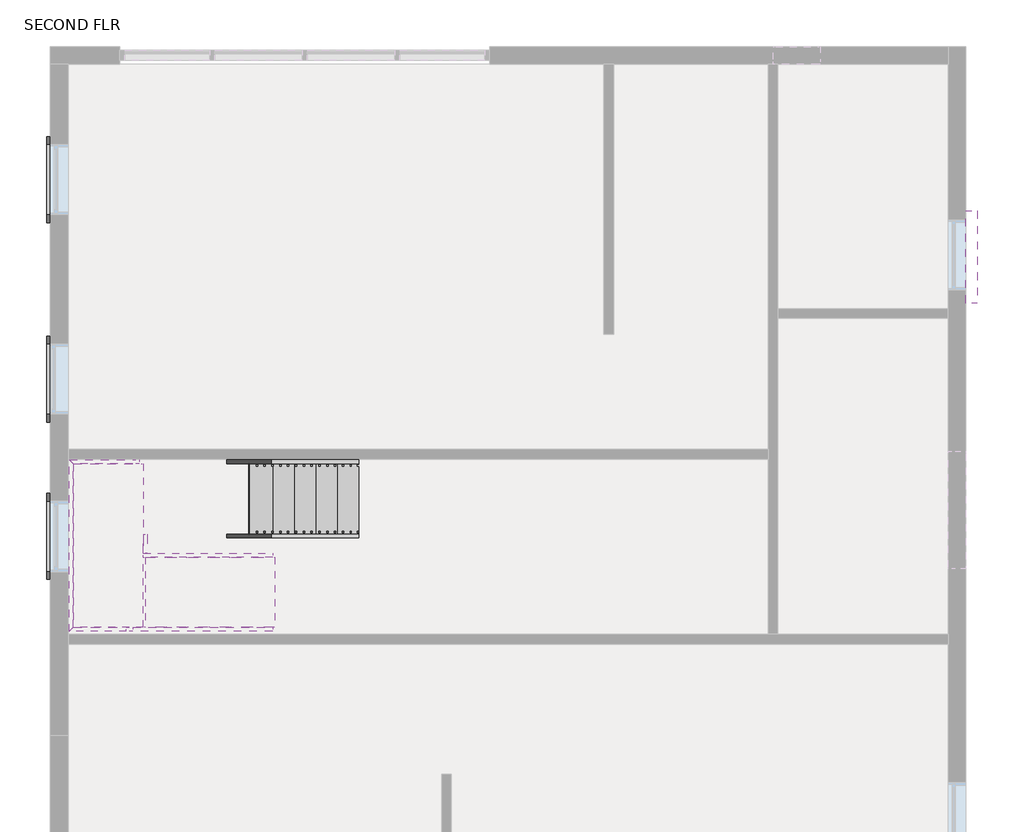
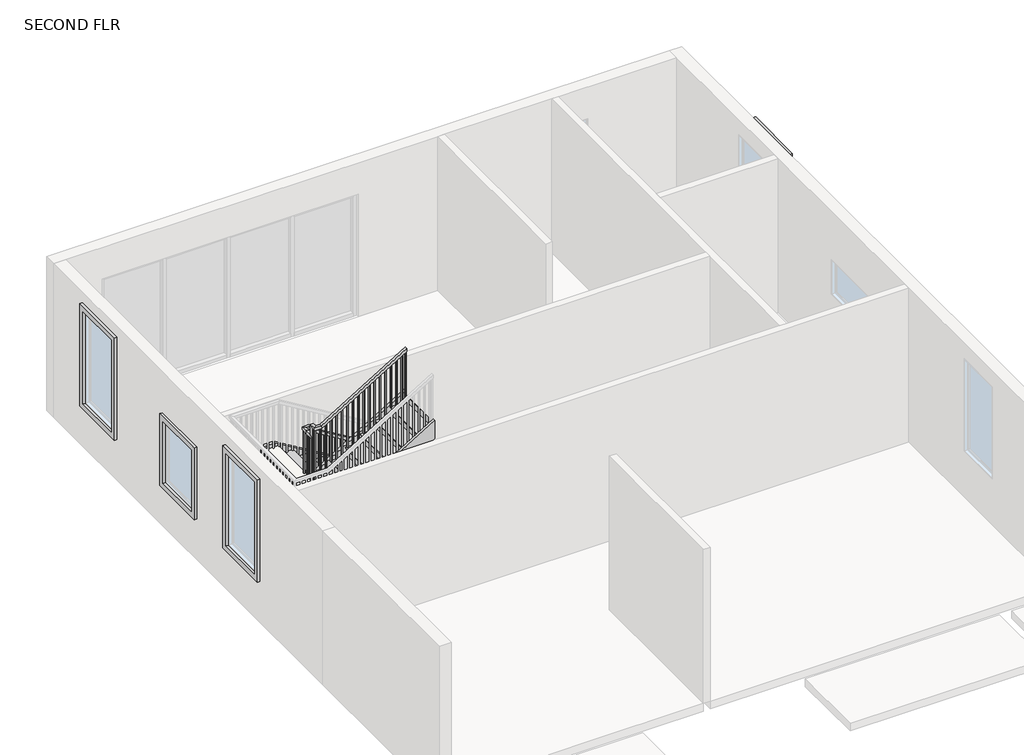
# One storey, part 3 of 3: 8 members, 4 proxies, 2 stair flights, 1 railing, 1 slab.
"""IFC4 building model written with IfcOpenShell, lengths in millimetres."""

from ifc_helpers import new_model, si_unit, frame, origin, place, context, project, spatial, polyline, outline, extrude, faceted_brep, transform, mapped, element, save
from components import generic_models_14_generic_models_13_4ffb657b, generic_models_21_generic_models_23_029173b4, generic_models_24_generic_models_24_8205a677, non_monolithic_landing_255cec53, stair_flight_4502834e, stair_flight_848efa21

model = new_model("IFC4")

# Units and contexts
model_context = context("Model", 3, world=origin())
ifc_project = project(units=[si_unit("LENGTHUNIT", "METRE", prefix="MILLI")], contexts=[model_context])

# Site, building, storey
site = spatial("IfcSite", under=ifc_project)
building = spatial("IfcBuilding", under=site)
storey = spatial("IfcBuildingStorey", under=building, Name="SECOND FLR", Elevation=6400.8)

# Proxies
placement = place(None, origin())
generic_models_14_generic_models_13_shape = generic_models_14_generic_models_13_4ffb657b(model_context)
element("IfcBuildingElementProxy", 1, Name="Generic Models 14 : Generic Models 13", ObjectType="Generic Models 14 : Generic Models 13", at=placement, inside=storey, context=model_context, shape_type="MappedRepresentation", body=[
    mapped(generic_models_14_generic_models_13_shape, transform((0.0, 7315.2, 0.0), x_axis=(1.0, 0.0, 0.0), y_axis=(0.0, 1.0, 0.0), z_axis=(0.0, 0.0, 1.0))),
])
generic_models_21_generic_models_23_shape = generic_models_21_generic_models_23_029173b4(model_context)
element("IfcBuildingElementProxy", 2, Name="Generic Models 23 : Generic Models 23", ObjectType="Generic Models 23 : Generic Models 23", at=placement, inside=storey, context=model_context, shape_type="MappedRepresentation", body=[
    mapped(generic_models_21_generic_models_23_shape, transform((0.0, 0.0, 0.0), x_axis=(1.0, 0.0, 0.0), y_axis=(0.0, 1.0, 0.0), z_axis=(0.0, 0.0, 1.0))),
])
generic_models_24_generic_models_24_shape = generic_models_24_generic_models_24_8205a677(model_context)
element("IfcBuildingElementProxy", 3, Name="Generic Models 24 : Generic Models 24", ObjectType="Generic Models 24 : Generic Models 24", at=placement, inside=storey, context=model_context, shape_type="MappedRepresentation", body=[
    mapped(generic_models_24_generic_models_24_shape, transform((0.0, 0.0, 0.0), x_axis=(1.0, 0.0, 0.0), y_axis=(0.0, 1.0, 0.0), z_axis=(0.0, 0.0, 1.0))),
])
element("IfcBuildingElementProxy", 4, Name="Generic Models 27 : Generic Models 23", ObjectType="Generic Models 27 : Generic Models 23", at=placement, inside=storey, context=model_context, shape_type="MappedRepresentation", body=[
    mapped(generic_models_21_generic_models_23_shape, transform((0.0, -4635.5, 0.0), x_axis=(1.0, 0.0, 0.0), y_axis=(0.0, 1.0, 0.0), z_axis=(0.0, 0.0, 1.0))),
])

# Members
element("IfcMember", 5, ObjectType="Stringer - 2\" Width", at=placement, inside=storey, context=model_context, shape_type="SweptSolid", body=[
    extrude(outline(polyline([(6705.6, -5990.8517085), (6917.714512, -5990.8517085), (8580.2599665, -8734.0517085), (8223.851205, -8734.0517085), (6705.6, -6228.9372203), (6705.6, -5990.8517085)])), frame((0.0, 1953.8826226, 0.0), z_axis=(0.0, 1.0, 0.0), x_axis=(0.0, 0.0, 1.0)), (0.0, 0.0, 1.0), 50.8),
])
element("IfcMember", 6, ObjectType="Stringer - 2\" Width", at=placement, inside=storey, context=model_context, shape_type="SweptSolid", body=[
    extrude(outline(polyline([(6705.6, -5990.8517085), (6917.714512, -5990.8517085), (8644.4666667, -8839.9927638), (8339.6666667, -8925.1472203), (6705.6, -6228.9372203), (6705.6, -5990.8517085)])), frame((0.0, 2919.0826226, 0.0), z_axis=(0.0, 1.0, 0.0), x_axis=(0.0, 0.0, 1.0)), (0.0, 0.0, 1.0), 50.8),
])
element("IfcMember", 7, ObjectType="Stringer - 2\" Width", at=placement, inside=storey, context=model_context, shape_type="SweptSolid", body=[
    extrude(outline(polyline([(8780.3811786, -8784.8517085), (8423.9724171, -8784.8517085), (9439.9724171, -7108.4517085), (9796.3811786, -7108.4517085), (8780.3811786, -8784.8517085)])), frame((0.0, 1706.4165128, 0.0), z_axis=(0.0, 1.0, 0.0), x_axis=(0.0, 0.0, 1.0)), (0.0, 0.0, 1.0), 50.8),
])
element("IfcMember", 8, ObjectType="Stringer - 2\" Width", at=placement, inside=storey, context=model_context, shape_type="SweptSolid", body=[
    extrude(outline(polyline([(8644.4666667, -9009.1106533), (8339.6666667, -8923.9561967), (9439.9724171, -7108.4517085), (9796.3811786, -7108.4517085), (8644.4666667, -9009.1106533)])), frame((0.0, 741.2165128, 0.0), z_axis=(0.0, 1.0, 0.0), x_axis=(0.0, 0.0, 1.0)), (0.0, 0.0, 1.0), 50.8),
])
element("IfcMember", 9, ObjectType="Stringer - 2\" Width", at=placement, inside=storey, context=model_context, shape_type="SweptSolid", body=[
    extrude(outline(polyline([(-8734.0517085, 1757.2165128), (-8784.8517085, 1757.2165128), (-8784.8517085, 2004.6826226), (-8734.0517085, 2004.6826226), (-8734.0517085, 1757.2165128)])), frame((0.0, 0.0, 8339.6666667), z_axis=(0.0, 0.0, 1.0), x_axis=(1.0, 0.0, 0.0)), (0.0, 0.0, 1.0), 304.8),
])
element("IfcMember", 10, ObjectType="Stringer - 2\" Width", at=placement, inside=storey, context=model_context, shape_type="Brep", body=[
    faceted_brep([(-8839.9927638, 2919.0826226, 8644.4666667), (-8839.9927638, 2969.8826226, 8644.4666667), (-9750.0517085, 2969.8826226, 8644.4666667), (-9699.2517085, 2919.0826226, 8644.4666667), (-8925.1472203, 2919.0826226, 8339.6666667), (-9699.2517085, 2919.0826226, 8339.6666667), (-8925.1472203, 2969.8826226, 8339.6666667), (-9750.0517085, 2969.8826226, 8339.6666667)], [[[0, 1, 2, 3]], [[4, 0, 3, 5]], [[6, 4, 5, 7]], [[1, 6, 7, 2]], [[1, 0, 4, 6]], [[2, 7, 5, 3]]]),
])
element("IfcMember", 11, ObjectType="Stringer - 2\" Width", at=placement, inside=storey, context=model_context, shape_type="SweptSolid", body=[
    extrude(outline(polyline([(-9750.0517085, 2969.8826226), (-9699.2517085, 2919.0826226), (-9699.2517085, 792.0165128), (-9750.0517085, 741.2165128), (-9750.0517085, 2969.8826226)])), frame((0.0, 0.0, 8339.6666667), z_axis=(0.0, 0.0, 1.0), x_axis=(1.0, 0.0, 0.0)), (0.0, 0.0, 1.0), 304.8),
])
element("IfcMember", 12, ObjectType="Stringer - 2\" Width", at=placement, inside=storey, context=model_context, shape_type="Brep", body=[
    faceted_brep([(-9699.2517085, 792.0165128, 8644.4666667), (-9750.0517085, 741.2165128, 8644.4666667), (-9009.1106533, 741.2165128, 8644.4666667), (-9009.1106533, 792.0165128, 8644.4666667), (-9699.2517085, 792.0165128, 8339.6666667), (-8923.9561967, 792.0165128, 8339.6666667), (-9750.0517085, 741.2165128, 8339.6666667), (-8923.9561967, 741.2165128, 8339.6666667)], [[[0, 1, 2, 3]], [[4, 0, 3, 5]], [[6, 4, 5, 7]], [[1, 6, 7, 2]], [[1, 0, 4, 6]], [[2, 7, 5, 3]]]),
])

# Railing
element("IfcRailing", 13, ObjectType="Handrail - Rectangular", at=placement, inside=storey, context=model_context, shape_type="SolidModel", body=[
    faceted_brep([(-5990.8517085, 2004.6826226, 7789.3333333), (-5990.8517085, 2004.6826226, 7729.9318731), (-5990.8517085, 2055.4826226, 7729.9318731), (-5990.8517085, 2055.4826226, 7789.3333333), (-8708.6517085, 2004.6826226, 9436.4848485), (-8759.4517085, 2004.6826226, 9407.871267), (-8759.4517085, 2055.4826226, 9407.871267), (-8708.6517085, 2055.4826226, 9436.4848485), (-8708.6517085, 2004.6826226, 9482.6666667), (-8759.4517085, 2004.6826226, 9431.8666667), (-8759.4517085, 2055.4826226, 9431.8666667), (-8708.6517085, 2055.4826226, 9482.6666667), (-8784.8517085, 2004.6826226, 9482.6666667), (-8784.8517085, 2004.6826226, 9431.8666667), (-8835.6517085, 2055.4826226, 9431.8666667), (-8835.6517085, 2055.4826226, 9482.6666667), (-8784.8517085, 1928.4826226, 9482.6666667), (-8784.8517085, 1928.4826226, 9431.8666667), (-8835.6517085, 1928.4826226, 9431.8666667), (-8835.6517085, 1928.4826226, 9482.6666667), (-8784.8517085, 1782.6165128, 9482.6666667), (-8784.8517085, 1731.8165128, 9431.8666667), (-8835.6517085, 1731.8165128, 9431.8666667), (-8835.6517085, 1782.6165128, 9482.6666667), (-8784.8517085, 1782.6165128, 9698.1818182), (-8784.8517085, 1731.8165128, 9647.3818182), (-8835.6517085, 1731.8165128, 9647.3818182), (-8835.6517085, 1782.6165128, 9698.1818182), (-8784.8517085, 1706.4165128, 9698.1818182), (-8784.8517085, 1706.4165128, 9647.3818182), (-8835.6517085, 1655.6165128, 9647.3818182), (-8835.6517085, 1655.6165128, 9698.1818182), (-8708.6517085, 1706.4165128, 9698.1818182), (-8694.4592991, 1706.4165128, 9647.3818182), (-8694.4592991, 1655.6165128, 9647.3818182), (-8708.6517085, 1655.6165128, 9698.1818182), (-7108.4517085, 1706.4165128, 10668.0), (-7108.4517085, 1655.6165128, 10668.0), (-7108.4517085, 1655.6165128, 10608.5985397), (-7108.4517085, 1706.4165128, 10608.5985397)], [[[0, 1, 2, 3]], [[1, 0, 4, 5]], [[2, 1, 5, 6]], [[3, 2, 6, 7]], [[0, 3, 7, 4]], [[5, 4, 8, 9]], [[6, 5, 9, 10]], [[7, 6, 10, 11]], [[4, 7, 11, 8]], [[9, 8, 12, 13]], [[10, 9, 13, 14]], [[11, 10, 14, 15]], [[8, 11, 15, 12]], [[13, 12, 16, 17]], [[14, 13, 17, 18]], [[15, 14, 18, 19]], [[12, 15, 19, 16]], [[17, 16, 20, 21]], [[18, 17, 21, 22]], [[19, 18, 22, 23]], [[16, 19, 23, 20]], [[21, 20, 24, 25]], [[22, 21, 25, 26]], [[23, 22, 26, 27]], [[20, 23, 27, 24]], [[25, 24, 28, 29]], [[26, 25, 29, 30]], [[27, 26, 30, 31]], [[24, 27, 31, 28]], [[29, 28, 32, 33]], [[30, 29, 33, 34]], [[31, 30, 34, 35]], [[28, 31, 35, 32]], [[36, 37, 38, 39]], [[33, 32, 36, 39]], [[34, 33, 39, 38]], [[35, 34, 38, 37]], [[32, 35, 37, 36]]]),
    extrude(outline(polyline([(10556.6439943, -7194.1767085), (9584.2666667, -7194.1767085), (9584.2666667, -7175.1267085), (10568.1894488, -7175.1267085), (10556.6439943, -7194.1767085)])), frame((0.0, 1671.4915128, 0.0), z_axis=(0.0, 1.0, 0.0), x_axis=(0.0, 0.0, 1.0)), (0.0, 0.0, 1.0), 19.05),
    extrude(outline(polyline([(10495.0682367, -7295.7767085), (9584.2666667, -7295.7767085), (9584.2666667, -7276.7267085), (10506.6136913, -7276.7267085), (10495.0682367, -7295.7767085)])), frame((0.0, 1671.4915128, 0.0), z_axis=(0.0, 1.0, 0.0), x_axis=(0.0, 0.0, 1.0)), (0.0, 0.0, 1.0), 19.05),
    extrude(outline(polyline([(10433.4924791, -7397.3767085), (9584.2666667, -7397.3767085), (9584.2666667, -7378.3267085), (10445.0379337, -7378.3267085), (10433.4924791, -7397.3767085)])), frame((0.0, 1671.4915128, 0.0), z_axis=(0.0, 1.0, 0.0), x_axis=(0.0, 0.0, 1.0)), (0.0, 0.0, 1.0), 19.05),
    extrude(outline(polyline([(10371.9167216, -7498.9767085), (9414.9333333, -7498.9767085), (9414.9333333, -7479.9267085), (10383.4621761, -7479.9267085), (10371.9167216, -7498.9767085)])), frame((0.0, 1671.4915128, 0.0), z_axis=(0.0, 1.0, 0.0), x_axis=(0.0, 0.0, 1.0)), (0.0, 0.0, 1.0), 19.05),
    extrude(outline(polyline([(10310.340964, -7600.5767085), (9414.9333333, -7600.5767085), (9414.9333333, -7581.5267085), (10321.8864185, -7581.5267085), (10310.340964, -7600.5767085)])), frame((0.0, 1671.4915128, 0.0), z_axis=(0.0, 1.0, 0.0), x_axis=(0.0, 0.0, 1.0)), (0.0, 0.0, 1.0), 19.05),
    extrude(outline(polyline([(10248.7652064, -7702.1767085), (9245.6, -7702.1767085), (9245.6, -7683.1267085), (10260.310661, -7683.1267085), (10248.7652064, -7702.1767085)])), frame((0.0, 1671.4915128, 0.0), z_axis=(0.0, 1.0, 0.0), x_axis=(0.0, 0.0, 1.0)), (0.0, 0.0, 1.0), 19.05),
    extrude(outline(polyline([(10187.1894488, -7803.7767085), (9245.6, -7803.7767085), (9245.6, -7784.7267085), (10198.7349034, -7784.7267085), (10187.1894488, -7803.7767085)])), frame((0.0, 1671.4915128, 0.0), z_axis=(0.0, 1.0, 0.0), x_axis=(0.0, 0.0, 1.0)), (0.0, 0.0, 1.0), 19.05),
    extrude(outline(polyline([(10125.6136913, -7905.3767085), (9245.6, -7905.3767085), (9245.6, -7886.3267085), (10137.1591458, -7886.3267085), (10125.6136913, -7905.3767085)])), frame((0.0, 1671.4915128, 0.0), z_axis=(0.0, 1.0, 0.0), x_axis=(0.0, 0.0, 1.0)), (0.0, 0.0, 1.0), 19.05),
    extrude(outline(polyline([(10064.0379337, -8006.9767085), (9076.2666667, -8006.9767085), (9076.2666667, -7987.9267085), (10075.5833882, -7987.9267085), (10064.0379337, -8006.9767085)])), frame((0.0, 1671.4915128, 0.0), z_axis=(0.0, 1.0, 0.0), x_axis=(0.0, 0.0, 1.0)), (0.0, 0.0, 1.0), 19.05),
    extrude(outline(polyline([(10002.4621761, -8108.5767085), (9076.2666667, -8108.5767085), (9076.2666667, -8089.5267085), (10014.0076307, -8089.5267085), (10002.4621761, -8108.5767085)])), frame((0.0, 1671.4915128, 0.0), z_axis=(0.0, 1.0, 0.0), x_axis=(0.0, 0.0, 1.0)), (0.0, 0.0, 1.0), 19.05),
    extrude(outline(polyline([(9940.8864185, -8210.1767085), (9076.2666667, -8210.1767085), (9076.2666667, -8191.1267085), (9952.4318731, -8191.1267085), (9940.8864185, -8210.1767085)])), frame((0.0, 1671.4915128, 0.0), z_axis=(0.0, 1.0, 0.0), x_axis=(0.0, 0.0, 1.0)), (0.0, 0.0, 1.0), 19.05),
    extrude(outline(polyline([(9879.310661, -8311.7767085), (8906.9333333, -8311.7767085), (8906.9333333, -8292.7267085), (9890.8561155, -8292.7267085), (9879.310661, -8311.7767085)])), frame((0.0, 1671.4915128, 0.0), z_axis=(0.0, 1.0, 0.0), x_axis=(0.0, 0.0, 1.0)), (0.0, 0.0, 1.0), 19.05),
    extrude(outline(polyline([(9817.7349034, -8413.3767085), (8906.9333333, -8413.3767085), (8906.9333333, -8394.3267085), (9829.2803579, -8394.3267085), (9817.7349034, -8413.3767085)])), frame((0.0, 1671.4915128, 0.0), z_axis=(0.0, 1.0, 0.0), x_axis=(0.0, 0.0, 1.0)), (0.0, 0.0, 1.0), 19.05),
    extrude(outline(polyline([(9756.1591458, -8514.9767085), (8906.9333333, -8514.9767085), (8906.9333333, -8495.9267085), (9767.7046004, -8495.9267085), (9756.1591458, -8514.9767085)])), frame((0.0, 1671.4915128, 0.0), z_axis=(0.0, 1.0, 0.0), x_axis=(0.0, 0.0, 1.0)), (0.0, 0.0, 1.0), 19.05),
    extrude(outline(polyline([(9694.5833882, -8616.5767085), (8737.6, -8616.5767085), (8737.6, -8597.5267085), (9706.1288428, -8597.5267085), (9694.5833882, -8616.5767085)])), frame((0.0, 1671.4915128, 0.0), z_axis=(0.0, 1.0, 0.0), x_axis=(0.0, 0.0, 1.0)), (0.0, 0.0, 1.0), 19.05),
    extrude(outline(polyline([(9633.0076307, -8718.1767085), (8737.6, -8718.1767085), (8737.6, -8699.1267085), (9644.5530852, -8699.1267085), (9633.0076307, -8718.1767085)])), frame((0.0, 1671.4915128, 0.0), z_axis=(0.0, 1.0, 0.0), x_axis=(0.0, 0.0, 1.0)), (0.0, 0.0, 1.0), 19.05),
    extrude(outline(polyline([(-8800.7267085, 1734.8076226), (-8800.7267085, 1715.7576226), (-8819.7767085, 1715.7576226), (-8819.7767085, 1734.8076226), (-8800.7267085, 1734.8076226)])), frame((0.0, 0.0, 8568.2666667), z_axis=(0.0, 0.0, 1.0), x_axis=(1.0, 0.0, 0.0)), (0.0, 0.0, 1.0), 1079.1151515),
    extrude(outline(polyline([(-8800.7267085, 1836.4076226), (-8800.7267085, 1817.3576226), (-8819.7767085, 1817.3576226), (-8819.7767085, 1836.4076226), (-8800.7267085, 1836.4076226)])), frame((0.0, 0.0, 8568.2666667), z_axis=(0.0, 0.0, 1.0), x_axis=(1.0, 0.0, 0.0)), (0.0, 0.0, 1.0), 863.6),
    extrude(outline(polyline([(-8800.7267085, 1938.0076226), (-8800.7267085, 1918.9576226), (-8819.7767085, 1918.9576226), (-8819.7767085, 1938.0076226), (-8800.7267085, 1938.0076226)])), frame((0.0, 0.0, 8568.2666667), z_axis=(0.0, 0.0, 1.0), x_axis=(1.0, 0.0, 0.0)), (0.0, 0.0, 1.0), 863.6),
    extrude(outline(polyline([(-8724.5267085, 2020.5576226), (-8743.5767085, 2020.5576226), (-8743.5767085, 2039.6076226), (-8724.5267085, 2039.6076226), (-8724.5267085, 2020.5576226)])), frame((0.0, 0.0, 8398.9333333), z_axis=(0.0, 0.0, 1.0), x_axis=(1.0, 0.0, 0.0)), (0.0, 0.0, 1.0), 1032.9333333),
    extrude(outline(polyline([(9336.6742973, -8641.9767085), (8398.9333333, -8641.9767085), (8398.9333333, -8622.9267085), (9325.1288428, -8622.9267085), (9336.6742973, -8641.9767085)])), frame((0.0, 2020.5576226, 0.0), z_axis=(0.0, 1.0, 0.0), x_axis=(0.0, 0.0, 1.0)), (0.0, 0.0, 1.0), 19.05),
    extrude(outline(polyline([(9275.0985397, -8540.3767085), (8398.9333333, -8540.3767085), (8398.9333333, -8521.3267085), (9263.5530852, -8521.3267085), (9275.0985397, -8540.3767085)])), frame((0.0, 2020.5576226, 0.0), z_axis=(0.0, 1.0, 0.0), x_axis=(0.0, 0.0, 1.0)), (0.0, 0.0, 1.0), 19.05),
    extrude(outline(polyline([(9213.5227822, -8438.7767085), (8229.6, -8438.7767085), (8229.6, -8419.7267085), (9201.9773276, -8419.7267085), (9213.5227822, -8438.7767085)])), frame((0.0, 2020.5576226, 0.0), z_axis=(0.0, 1.0, 0.0), x_axis=(0.0, 0.0, 1.0)), (0.0, 0.0, 1.0), 19.05),
    extrude(outline(polyline([(9151.9470246, -8337.1767085), (8229.6, -8337.1767085), (8229.6, -8318.1267085), (9140.40157, -8318.1267085), (9151.9470246, -8337.1767085)])), frame((0.0, 2020.5576226, 0.0), z_axis=(0.0, 1.0, 0.0), x_axis=(0.0, 0.0, 1.0)), (0.0, 0.0, 1.0), 19.05),
    extrude(outline(polyline([(9090.371267, -8235.5767085), (8229.6, -8235.5767085), (8229.6, -8216.5267085), (9078.8258125, -8216.5267085), (9090.371267, -8235.5767085)])), frame((0.0, 2020.5576226, 0.0), z_axis=(0.0, 1.0, 0.0), x_axis=(0.0, 0.0, 1.0)), (0.0, 0.0, 1.0), 19.05),
    extrude(outline(polyline([(9028.7955094, -8133.9767085), (8060.2666667, -8133.9767085), (8060.2666667, -8114.9267085), (9017.2500549, -8114.9267085), (9028.7955094, -8133.9767085)])), frame((0.0, 2020.5576226, 0.0), z_axis=(0.0, 1.0, 0.0), x_axis=(0.0, 0.0, 1.0)), (0.0, 0.0, 1.0), 19.05),
    extrude(outline(polyline([(8967.2197519, -8032.3767085), (8060.2666667, -8032.3767085), (8060.2666667, -8013.3267085), (8955.6742973, -8013.3267085), (8967.2197519, -8032.3767085)])), frame((0.0, 2020.5576226, 0.0), z_axis=(0.0, 1.0, 0.0), x_axis=(0.0, 0.0, 1.0)), (0.0, 0.0, 1.0), 19.05),
    extrude(outline(polyline([(8905.6439943, -7930.7767085), (7890.9333333, -7930.7767085), (7890.9333333, -7911.7267085), (8894.0985397, -7911.7267085), (8905.6439943, -7930.7767085)])), frame((0.0, 2020.5576226, 0.0), z_axis=(0.0, 1.0, 0.0), x_axis=(0.0, 0.0, 1.0)), (0.0, 0.0, 1.0), 19.05),
    extrude(outline(polyline([(8844.0682367, -7829.1767085), (7890.9333333, -7829.1767085), (7890.9333333, -7810.1267085), (8832.5227822, -7810.1267085), (8844.0682367, -7829.1767085)])), frame((0.0, 2020.5576226, 0.0), z_axis=(0.0, 1.0, 0.0), x_axis=(0.0, 0.0, 1.0)), (0.0, 0.0, 1.0), 19.05),
    extrude(outline(polyline([(8782.4924791, -7727.5767085), (7890.9333333, -7727.5767085), (7890.9333333, -7708.5267085), (8770.9470246, -7708.5267085), (8782.4924791, -7727.5767085)])), frame((0.0, 2020.5576226, 0.0), z_axis=(0.0, 1.0, 0.0), x_axis=(0.0, 0.0, 1.0)), (0.0, 0.0, 1.0), 19.05),
    extrude(outline(polyline([(8720.9167216, -7625.9767085), (7721.6, -7625.9767085), (7721.6, -7606.9267085), (8709.371267, -7606.9267085), (8720.9167216, -7625.9767085)])), frame((0.0, 2020.5576226, 0.0), z_axis=(0.0, 1.0, 0.0), x_axis=(0.0, 0.0, 1.0)), (0.0, 0.0, 1.0), 19.05),
    extrude(outline(polyline([(8659.340964, -7524.3767085), (7721.6, -7524.3767085), (7721.6, -7505.3267085), (8647.7955094, -7505.3267085), (8659.340964, -7524.3767085)])), frame((0.0, 2020.5576226, 0.0), z_axis=(0.0, 1.0, 0.0), x_axis=(0.0, 0.0, 1.0)), (0.0, 0.0, 1.0), 19.05),
    extrude(outline(polyline([(8597.7652064, -7422.7767085), (7721.6, -7422.7767085), (7721.6, -7403.7267085), (8586.2197519, -7403.7267085), (8597.7652064, -7422.7767085)])), frame((0.0, 2020.5576226, 0.0), z_axis=(0.0, 1.0, 0.0), x_axis=(0.0, 0.0, 1.0)), (0.0, 0.0, 1.0), 19.05),
    extrude(outline(polyline([(8536.1894488, -7321.1767085), (7552.2666667, -7321.1767085), (7552.2666667, -7302.1267085), (8524.6439943, -7302.1267085), (8536.1894488, -7321.1767085)])), frame((0.0, 2020.5576226, 0.0), z_axis=(0.0, 1.0, 0.0), x_axis=(0.0, 0.0, 1.0)), (0.0, 0.0, 1.0), 19.05),
    extrude(outline(polyline([(8474.6136913, -7219.5767085), (7552.2666667, -7219.5767085), (7552.2666667, -7200.5267085), (8463.0682367, -7200.5267085), (8474.6136913, -7219.5767085)])), frame((0.0, 2020.5576226, 0.0), z_axis=(0.0, 1.0, 0.0), x_axis=(0.0, 0.0, 1.0)), (0.0, 0.0, 1.0), 19.05),
    extrude(outline(polyline([(8413.0379337, -7117.9767085), (7552.2666667, -7117.9767085), (7552.2666667, -7098.9267085), (8401.4924791, -7098.9267085), (8413.0379337, -7117.9767085)])), frame((0.0, 2020.5576226, 0.0), z_axis=(0.0, 1.0, 0.0), x_axis=(0.0, 0.0, 1.0)), (0.0, 0.0, 1.0), 19.05),
    extrude(outline(polyline([(8351.4621761, -7016.3767085), (7382.9333333, -7016.3767085), (7382.9333333, -6997.3267085), (8339.9167216, -6997.3267085), (8351.4621761, -7016.3767085)])), frame((0.0, 2020.5576226, 0.0), z_axis=(0.0, 1.0, 0.0), x_axis=(0.0, 0.0, 1.0)), (0.0, 0.0, 1.0), 19.05),
    extrude(outline(polyline([(8289.8864185, -6914.7767085), (7382.9333333, -6914.7767085), (7382.9333333, -6895.7267085), (8278.340964, -6895.7267085), (8289.8864185, -6914.7767085)])), frame((0.0, 2020.5576226, 0.0), z_axis=(0.0, 1.0, 0.0), x_axis=(0.0, 0.0, 1.0)), (0.0, 0.0, 1.0), 19.05),
    extrude(outline(polyline([(8228.310661, -6813.1767085), (7213.6, -6813.1767085), (7213.6, -6794.1267085), (8216.7652064, -6794.1267085), (8228.310661, -6813.1767085)])), frame((0.0, 2020.5576226, 0.0), z_axis=(0.0, 1.0, 0.0), x_axis=(0.0, 0.0, 1.0)), (0.0, 0.0, 1.0), 19.05),
    extrude(outline(polyline([(8166.7349034, -6711.5767085), (7213.6, -6711.5767085), (7213.6, -6692.5267085), (8155.1894488, -6692.5267085), (8166.7349034, -6711.5767085)])), frame((0.0, 2020.5576226, 0.0), z_axis=(0.0, 1.0, 0.0), x_axis=(0.0, 0.0, 1.0)), (0.0, 0.0, 1.0), 19.05),
    extrude(outline(polyline([(8105.1591458, -6609.9767085), (7213.6, -6609.9767085), (7213.6, -6590.9267085), (8093.6136913, -6590.9267085), (8105.1591458, -6609.9767085)])), frame((0.0, 2020.5576226, 0.0), z_axis=(0.0, 1.0, 0.0), x_axis=(0.0, 0.0, 1.0)), (0.0, 0.0, 1.0), 19.05),
    extrude(outline(polyline([(8043.5833882, -6508.3767085), (7044.2666667, -6508.3767085), (7044.2666667, -6489.3267085), (8032.0379337, -6489.3267085), (8043.5833882, -6508.3767085)])), frame((0.0, 2020.5576226, 0.0), z_axis=(0.0, 1.0, 0.0), x_axis=(0.0, 0.0, 1.0)), (0.0, 0.0, 1.0), 19.05),
    extrude(outline(polyline([(7982.0076307, -6406.7767085), (7044.2666667, -6406.7767085), (7044.2666667, -6387.7267085), (7970.4621761, -6387.7267085), (7982.0076307, -6406.7767085)])), frame((0.0, 2020.5576226, 0.0), z_axis=(0.0, 1.0, 0.0), x_axis=(0.0, 0.0, 1.0)), (0.0, 0.0, 1.0), 19.05),
    extrude(outline(polyline([(7920.4318731, -6305.1767085), (7044.2666667, -6305.1767085), (7044.2666667, -6286.1267085), (7908.8864185, -6286.1267085), (7920.4318731, -6305.1767085)])), frame((0.0, 2020.5576226, 0.0), z_axis=(0.0, 1.0, 0.0), x_axis=(0.0, 0.0, 1.0)), (0.0, 0.0, 1.0), 19.05),
    extrude(outline(polyline([(7858.8561155, -6203.5767085), (6874.9333333, -6203.5767085), (6874.9333333, -6184.5267085), (7847.310661, -6184.5267085), (7858.8561155, -6203.5767085)])), frame((0.0, 2020.5576226, 0.0), z_axis=(0.0, 1.0, 0.0), x_axis=(0.0, 0.0, 1.0)), (0.0, 0.0, 1.0), 19.05),
    extrude(outline(polyline([(7797.2803579, -6101.9767085), (6874.9333333, -6101.9767085), (6874.9333333, -6082.9267085), (7785.7349034, -6082.9267085), (7797.2803579, -6101.9767085)])), frame((0.0, 2020.5576226, 0.0), z_axis=(0.0, 1.0, 0.0), x_axis=(0.0, 0.0, 1.0)), (0.0, 0.0, 1.0), 19.05),
    extrude(outline(polyline([(-8800.7267085, 1690.5415128), (-8800.7267085, 1671.4915128), (-8819.7767085, 1671.4915128), (-8819.7767085, 1690.5415128), (-8800.7267085, 1690.5415128)])), frame((0.0, 0.0, 8568.2666667), z_axis=(0.0, 0.0, 1.0), x_axis=(1.0, 0.0, 0.0)), (0.0, 0.0, 1.0), 1079.1151515),
    extrude(outline(polyline([(-8800.7267085, 2020.5576226), (-8819.7767085, 2020.5576226), (-8819.7767085, 2039.6076226), (-8800.7267085, 2039.6076226), (-8800.7267085, 2020.5576226)])), frame((0.0, 0.0, 8568.2666667), z_axis=(0.0, 0.0, 1.0), x_axis=(1.0, 0.0, 0.0)), (0.0, 0.0, 1.0), 863.6),
    extrude(outline(polyline([(10597.0530852, -7127.5017085), (9584.2666667, -7127.5017085), (9584.2666667, -7108.4517085), (10608.5985397, -7108.4517085), (10597.0530852, -7127.5017085)])), frame((0.0, 1671.4915128, 0.0), z_axis=(0.0, 1.0, 0.0), x_axis=(0.0, 0.0, 1.0)), (0.0, 0.0, 1.0), 19.05),
    extrude(outline(polyline([(7741.4773276, -6009.9017085), (6874.9333333, -6009.9017085), (6874.9333333, -5990.8517085), (7729.9318731, -5990.8517085), (7741.4773276, -6009.9017085)])), frame((0.0, 2020.5576226, 0.0), z_axis=(0.0, 1.0, 0.0), x_axis=(0.0, 0.0, 1.0)), (0.0, 0.0, 1.0), 19.05),
])

# Slab
non_monolithic_landing_shape = non_monolithic_landing_255cec53(model_context)
element("IfcSlab", 14, ObjectType="Non-Monolithic Landing", at=placement, inside=storey, context=model_context, shape_type="MappedRepresentation", body=[
    mapped(non_monolithic_landing_shape, transform((0.0, 0.0, 0.0), x_axis=(1.0, 0.0, 0.0), y_axis=(0.0, 1.0, 0.0), z_axis=(0.0, 0.0, 1.0))),
])

# Stair flights
stair_flight_shape = stair_flight_4502834e(model_context)
element("IfcStairFlight", 15, ObjectType="2\" Tread 1\" Nosing 1/4\" Riser", at=placement, inside=storey, context=model_context, shape_type="MappedRepresentation", body=[
    mapped(stair_flight_shape, transform((0.0, 0.0, 0.0), x_axis=(1.0, 0.0, 0.0), y_axis=(0.0, 1.0, 0.0), z_axis=(0.0, 0.0, 1.0))),
])
stair_flight_2_shape = stair_flight_848efa21(model_context)
element("IfcStairFlight", 16, ObjectType="2\" Tread 1\" Nosing 1/4\" Riser", at=placement, inside=storey, context=model_context, shape_type="MappedRepresentation", body=[
    mapped(stair_flight_2_shape, transform((0.0, 0.0, 0.0), x_axis=(1.0, 0.0, 0.0), y_axis=(0.0, 1.0, 0.0), z_axis=(0.0, 0.0, 1.0))),
])

save(model, "model.ifc")

# Revit data of these elements
# Type "Handrail - Rectangular"
#   Assembly Code = "C2010400"
#   built-in parameter 1008612 = 0.0416667 (stored number, unit not read)
#   built-in parameter 1008611 = 0.0416667 (stored number, unit not read)
#   built-in parameter 1008609 = 0.333333 (stored number, unit not read)
#   built-in parameter 1008604 = 0.166667 (stored number, unit not read)
#   built-in parameter 1008603 = 0.166667 (stored number, unit not read)
#   Railing Height = 3' - 0"
#   built-in parameter 1008630 = 2
#   built-in parameter 1008610 = 2
#   built-in parameter 1008618 = Baluster - Square : 3/4"
# Element 1 (IfcBuildingElementProxy, "Generic Models 14 : Generic Models 13")
#   Phase Created = New Construction
# Element 2 (IfcBuildingElementProxy, "Generic Models 23 : Generic Models 23")
#   Phase Created = New Construction
# Element 3 (IfcBuildingElementProxy, "Generic Models 24 : Generic Models 24")
#   Phase Created = New Construction
# Element 4 (IfcBuildingElementProxy, "Generic Models 27 : Generic Models 23")
#   Phase Created = New Construction
# Elements 5, 6, 7, 8, 9, 10, 11, 12 (IfcMember, "Stringer - 2\" Width")
#   Phase Created = New Construction
# Element 13 (IfcRailing, "Handrail - Rectangular")
#   Phase Created = New Construction
# Element 14 (IfcSlab, "Non-Monolithic Landing")
#   Phase Created = New Construction
# Elements 15, 16 (IfcStairFlight, "2\" Tread 1\" Nosing 1/4\" Riser")
#   Phase Created = New Construction
